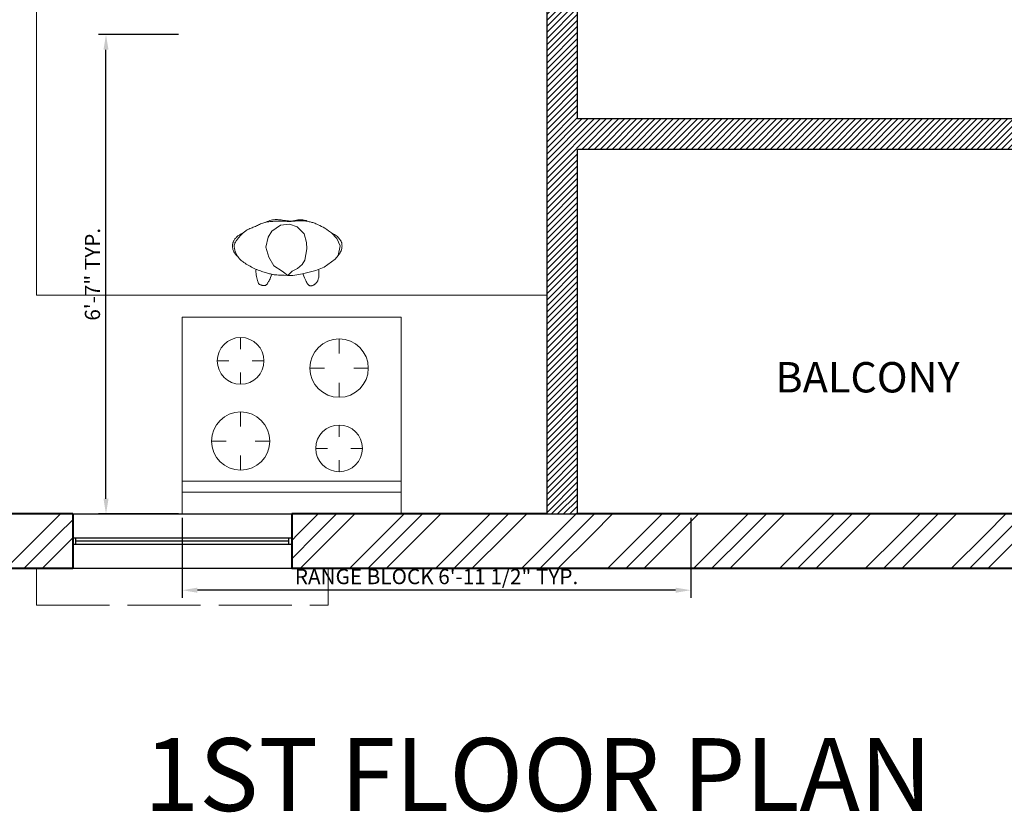
# Model space of a CAD drawing. Units: inches. Extents: x 2443635 to 2446153, y 1826255 to 1827341.
# Tile 7 of 16: x 2444366 to 2444528, y 1826821 to 1826952. Entities that reach past the tile are written whole.
import ezdxf

# ---------------------------------------------------------------- set-up
doc = ezdxf.new("R2010")
doc.units = ezdxf.units.IN
doc.linetypes.add('ACAD_ISO02W100', pattern=[15, 12, -3])
for name, color, linetype, lineweight in [('A-DIMS', 1, 'Continuous', 18), ('A-ENTG', 111, 'Continuous', 13), ('A-EQPM', 8, 'Continuous', 18), ('A-FLOR-CASE', 8, 'Continuous', 18), ('A-ROOM', 4, 'Continuous', 18), ('A-TEXT', 4, 'Continuous', 25), ('A-WALL-EXT', 7, 'Continuous', 40), ('A-WALL-INT', 9, 'Continuous', 30), ('A-WALL-OVHD', 7, 'ACAD_ISO02W100', 18), ('A-WALL-PATT', 8, 'Continuous', 13), ('A-WINDOW', 4, 'Continuous', 25)]:
    doc.layers.add(name, color=color, linetype=linetype, lineweight=lineweight)
doc.styles.add('ATT', font='romans.shx')
doc.styles.get("Standard").update_dxf_attribs({"font": 'arial.ttf'})
doc.dimstyles.new('ISO-25', dxfattribs={"dimtxt": 2.5, "dimasz": 2.5, "dimexe": 1.25, "dimexo": 0.625, "dimtad": 1, "dimlunit": 4, "dimtxsty": 'Standard', "dimcen": 2.5, "dimadec": 0, "dimazin": 0, "dimtfac": 1, "dimtmove": 0, "dimatfit": 3, "dimfxl": 1, "dimarcsym": 0})

# ---------------------------------------------------------------- blocks, each defined once
blk = doc.blocks.new('11PRNG01')
at = {"color": 0, "linetype": 'ByBlock'}
for p, q in [((0, 30), (27, 30)), ((0, 0), (0, 30)), ((3, 0), (3, 30)), ((4.5, 0), (4.5, 30)), ((27, 30), (27, 0)), ((10, 26), (10, 24)), ((21, 25.2), (21, 23.6)), ((6, 22), (8, 22)), ((14, 22), (12, 22)), ((17.8, 22), (19.4, 22)), ((24.2, 22), (22.6, 22)), ((21, 18.8), (21, 20.4)), ((10, 18), (10, 20)), ((20, 12.5), (20, 10.5)), ((9, 11.7), (9, 10.1)), ((5.8, 8.5), (7.4, 8.5)), ((12.2, 8.5), (10.6, 8.5)), ((16, 8.5), (18, 8.5)), ((24, 8.5), (22, 8.5)), ((9, 5.3), (9, 6.9)), ((20, 4.5), (20, 6.5)), ((27, 0), (0, 0))]:
    blk.add_line(p, q, dxfattribs=at)
for centre, radius in [((10, 22), 4), ((21, 22), 3.2), ((20, 8.5), 4), ((9, 8.5), 3.2)]:
    blk.add_circle(centre, radius, dxfattribs=at)
at = {"color": 0, "linetype": 'ByBlock', "style": 'ATT'}
for tag, p, flags in [('ITEM', (0, -11), 3), ('ROOM_NUMBER', (0, -20), 1), ('DEPTH', (0, -29), 3), ('WIDTH', (0, -38), 3)]:
    blk.add_attdef(tag, p, '', height=6, dxfattribs=dict(at, flags=flags))
blk = doc.blocks.new('PERSON-STANDING-PLAN')
at = {"transparency": 33554687}
for p, q in [((3.58, 9.72), (3.76, 9.79)), ((3.76, 9.79), (3.94, 9.87)), ((3.94, 9.87), (4.11, 9.95)), ((4.11, 9.95), (4.28, 10.02)), ((4.28, 10.02), (4.45, 10.1)), ((4.45, 10.1), (4.62, 10.18)), ((4.62, 10.18), (4.79, 10.25)), ((4.79, 10.25), (4.96, 10.31)), ((4.96, 10.31), (5.14, 10.38)), ((5.14, 10.38), (5.33, 10.43)), ((5.33, 10.43), (5.53, 10.48)), ((5.48, 10.5), (5.36, 10.44)), ((5.69, 10.59), (5.48, 10.5)), ((5.53, 10.48), (5.74, 10.51)), ((5.91, 10.67), (5.69, 10.59)), ((5.74, 10.51), (5.95, 10.55)), ((6.13, 10.74), (5.91, 10.67)), ((5.95, 10.55), (6.17, 10.57)), ((6.35, 10.79), (6.13, 10.74)), ((6.17, 10.57), (6.39, 10.59)), ((6.57, 10.84), (6.35, 10.79)), ((6.39, 10.59), (6.61, 10.61)), ((7.91, 9.98), (6.48, 9.01)), ((6.79, 10.87), (6.57, 10.84)), ((6.61, 10.61), (6.83, 10.62)), ((6.99, 10.89), (6.79, 10.87)), ((6.83, 10.62), (7.05, 10.63)), ((7.18, 10.9), (6.99, 10.89)), ((7.05, 10.63), (7.26, 10.64)), ((7.38, 10.9), (7.18, 10.9)), ((7.26, 10.64), (7.47, 10.65)), ((7.57, 10.88), (7.38, 10.9)), ((7.47, 10.65), (7.68, 10.65)), ((7.78, 10.87), (7.57, 10.88)), ((7.68, 10.65), (7.87, 10.65)), ((7.99, 10.84), (7.78, 10.87)), ((7.87, 10.65), (8.06, 10.65)), ((9.39, 10.13), (7.91, 9.98)), ((8.22, 10.82), (7.99, 10.84)), ((8.06, 10.65), (8.23, 10.65)), ((9.71, 10.64), (8.22, 10.82)), ((8.23, 10.65), (8.39, 10.65)), ((8.39, 10.65), (8.54, 10.64)), ((8.54, 10.64), (8.67, 10.64)), ((8.67, 10.64), (8.78, 10.63)), ((8.78, 10.63), (8.89, 10.62)), ((8.89, 10.62), (8.98, 10.61)), ((8.98, 10.61), (9.08, 10.6)), ((9.08, 10.6), (9.16, 10.59)), ((9.16, 10.59), (9.25, 10.59)), ((9.25, 10.59), (9.35, 10.59)), ((9.35, 10.59), (9.44, 10.59)), ((10.63, 9.72), (9.39, 10.13)), ((9.44, 10.59), (9.55, 10.6)), ((9.55, 10.6), (9.66, 10.61)), ((9.9, 10.69), (9.56, 10.61)), ((9.66, 10.61), (9.78, 10.62)), ((9.78, 10.62), (9.9, 10.63)), ((10.22, 10.76), (9.9, 10.69)), ((9.9, 10.63), (10.03, 10.64)), ((10.03, 10.64), (10.16, 10.66)), ((10.16, 10.66), (10.3, 10.67)), ((10.5, 10.81), (10.22, 10.76)), ((10.3, 10.67), (10.45, 10.68)), ((10.45, 10.68), (10.61, 10.7)), ((10.76, 10.84), (10.5, 10.81)), ((10.61, 10.7), (10.76, 10.71)), ((10.99, 10.86), (10.76, 10.84)), ((10.76, 10.71), (10.92, 10.71)), ((10.92, 10.71), (11.09, 10.72)), ((11.2, 10.87), (10.99, 10.86)), ((11.09, 10.72), (11.25, 10.72)), ((11.4, 10.86), (11.2, 10.87)), ((11.25, 10.72), (11.41, 10.72)), ((11.58, 10.84), (11.4, 10.86)), ((11.41, 10.72), (11.57, 10.71)), ((11.57, 10.71), (11.73, 10.7)), ((11.76, 10.81), (11.58, 10.84)), ((11.73, 10.7), (11.89, 10.68)), ((11.93, 10.77), (11.76, 10.81)), ((11.89, 10.68), (12.04, 10.67)), ((12.11, 10.73), (11.93, 10.77)), ((12.04, 10.67), (12.19, 10.64)), ((12.29, 10.67), (12.11, 10.73)), ((12.19, 10.64), (12.34, 10.62)), ((12.48, 10.61), (12.29, 10.67)), ((12.34, 10.62), (12.48, 10.59)), ((12.68, 10.55), (12.48, 10.61)), ((12.48, 10.59), (12.62, 10.56)), ((12.62, 10.56), (12.77, 10.53)), ((12.91, 10.49), (12.68, 10.55)), ((12.77, 10.53), (12.91, 10.49)), ((12.91, 10.49), (13.05, 10.45)), ((13.17, 10.43), (12.91, 10.49)), ((13.05, 10.45), (13.2, 10.41)), ((13.2, 10.41), (13.35, 10.36)), ((13.35, 10.36), (13.51, 10.3)), ((13.51, 10.3), (13.69, 10.22)), ((13.69, 10.22), (13.89, 10.14)), ((13.89, 10.14), (14.11, 10.04)), ((14.11, 10.04), (14.35, 9.93)), ((14.35, 9.93), (14.61, 9.79)), ((14.61, 9.79), (14.89, 9.64)), ((0.77, 8.12), (0.67, 8.02)), ((0.87, 8.21), (0.77, 8.12)), ((0.97, 8.29), (0.87, 8.21)), ((1.08, 8.36), (0.97, 8.29)), ((1.17, 8.42), (1.08, 8.36)), ((1.12, 8.07), (1.21, 8.17)), ((1.26, 8.47), (1.17, 8.42)), ((1.21, 8.17), (1.3, 8.27)), ((1.35, 8.51), (1.26, 8.47)), ((1.3, 8.27), (1.39, 8.37)), ((1.43, 8.54), (1.35, 8.51)), ((1.39, 8.37), (1.49, 8.47)), ((1.49, 8.56), (1.43, 8.54)), ((1.55, 8.58), (1.49, 8.56)), ((1.49, 8.47), (1.59, 8.57)), ((1.59, 8.59), (1.55, 8.58)), ((1.59, 8.57), (1.69, 8.66)), ((1.62, 8.6), (1.59, 8.59)), ((1.69, 8.66), (1.79, 8.76)), ((1.79, 8.76), (1.9, 8.85)), ((1.9, 8.85), (2.01, 8.94)), ((2.01, 8.94), (2.13, 9.02)), ((2.13, 9.02), (2.26, 9.11)), ((2.26, 9.11), (2.39, 9.19)), ((2.39, 9.19), (2.54, 9.27)), ((2.54, 9.27), (2.7, 9.35)), ((2.7, 9.35), (2.86, 9.42)), ((2.86, 9.42), (3.04, 9.5)), ((3.04, 9.5), (3.21, 9.57)), ((3.21, 9.57), (3.39, 9.65)), ((3.39, 9.65), (3.58, 9.72)), ((6.48, 9.01), (5.88, 8.02)), ((11.79, 8.58), (10.63, 9.72)), ((12.18, 7.14), (11.79, 8.58)), ((14.89, 9.64), (15.18, 9.47)), ((15.18, 9.47), (15.49, 9.28)), ((15.49, 9.28), (15.8, 9.07)), ((15.8, 9.07), (16.12, 8.84)), ((16.12, 8.84), (16.44, 8.59)), ((16.26, 8.74), (17.17, 7.78)), ((16.44, 8.59), (16.61, 8.53)), ((16.61, 8.53), (16.77, 8.45)), ((16.77, 8.45), (16.94, 8.35)), ((16.94, 8.35), (17.1, 8.23)), ((17.1, 8.23), (17.24, 8.1)), ((0.01, 6.79), (0, 6.71)), ((0, 6.71), (0, 6.61)), ((0, 6.61), (0, 6.52)), ((0, 6.52), (0, 6.42)), ((0.02, 6.88), (0.01, 6.79)), ((0.04, 6.97), (0.02, 6.88)), ((0.06, 7.06), (0.04, 6.97)), ((0.08, 7.15), (0.06, 7.06)), ((0.11, 7.23), (0.08, 7.15)), ((0.15, 7.33), (0.11, 7.23)), ((0.2, 7.42), (0.15, 7.33)), ((0.25, 7.51), (0.2, 7.42)), ((0.32, 7.61), (0.25, 7.51)), ((0.28, 6.52), (0.29, 6.66)), ((0.29, 6.38), (0.28, 6.52)), ((0.29, 6.66), (0.31, 6.8)), ((0.31, 6.8), (0.35, 6.93)), ((0.39, 7.71), (0.32, 7.61)), ((0.35, 6.93), (0.4, 7.06)), ((0.48, 7.82), (0.39, 7.71)), ((0.4, 7.06), (0.46, 7.18)), ((0.46, 7.18), (0.52, 7.3)), ((0.57, 7.92), (0.48, 7.82)), ((0.52, 7.3), (0.6, 7.41)), ((0.67, 8.02), (0.57, 7.92)), ((0.6, 7.41), (0.68, 7.53)), ((0.68, 7.53), (0.76, 7.64)), ((0.76, 7.64), (0.85, 7.75)), ((0.85, 7.75), (0.94, 7.85)), ((0.94, 7.85), (1.03, 7.96)), ((1.03, 7.96), (1.12, 8.07)), ((5.88, 8.02), (5.48, 6.38)), ((12.22, 6.07), (12.18, 7.14)), ((17.17, 7.78), (17.68, 6.58)), ((17.24, 8.1), (17.38, 7.96)), ((17.68, 6.58), (17.36, 5.01)), ((17.38, 7.96), (17.51, 7.82)), ((17.51, 7.82), (17.61, 7.69)), ((17.61, 7.69), (17.7, 7.56)), ((17.7, 7.56), (17.78, 7.45)), ((17.78, 7.45), (17.84, 7.34)), ((17.84, 7.34), (17.88, 7.24)), ((17.88, 7.24), (17.92, 7.15)), ((17.92, 7.15), (17.95, 7.06)), ((17.95, 7.06), (17.97, 6.97)), ((17.97, 6.97), (17.98, 6.88)), ((17.98, 6.88), (17.99, 6.79)), ((17.99, 6.79), (18, 6.71)), ((18, 6.71), (18.01, 6.61)), ((18.01, 6.52), (18, 6.42)), ((18.01, 6.61), (18.01, 6.52)), ((0, 6.42), (0.01, 6.33)), ((0.01, 6.33), (0.02, 6.22)), ((0.02, 6.22), (0.04, 6.12)), ((0.04, 6.12), (0.06, 6)), ((0.06, 6), (0.1, 5.88)), ((0.1, 5.88), (0.15, 5.75)), ((0.15, 5.75), (0.23, 5.6)), ((0.23, 5.6), (0.33, 5.43)), ((0.3, 6.24), (0.29, 6.38)), ((0.32, 6.09), (0.3, 6.24)), ((0.35, 5.95), (0.32, 6.09)), ((0.33, 5.43), (0.48, 5.23)), ((0.39, 5.81), (0.35, 5.95)), ((0.43, 5.68), (0.39, 5.81)), ((0.48, 5.55), (0.43, 5.68)), ((0.53, 5.42), (0.48, 5.55)), ((0.48, 5.23), (0.67, 5.01)), ((0.58, 5.3), (0.53, 5.42)), ((0.64, 5.19), (0.58, 5.3)), ((0.7, 5.07), (0.64, 5.19)), ((0.67, 5.01), (0.91, 4.75)), ((0.77, 4.96), (0.7, 5.07)), ((0.85, 4.85), (0.77, 4.96)), ((5.48, 6.38), (5.95, 4.72)), ((11.9, 4.25), (12.22, 6.07)), ((17.36, 5.01), (16.88, 4.4)), ((17.36, 5), (17.14, 4.74)), ((17.54, 5.23), (17.36, 5)), ((17.68, 5.42), (17.54, 5.23)), ((17.78, 5.6), (17.68, 5.42)), ((17.86, 5.75), (17.78, 5.6)), ((17.91, 5.88), (17.86, 5.75)), ((17.94, 6), (17.91, 5.88)), ((17.96, 6.12), (17.94, 6)), ((17.98, 6.22), (17.96, 6.12)), ((17.99, 6.33), (17.98, 6.22)), ((18, 6.42), (17.99, 6.33)), ((0.93, 4.74), (0.85, 4.85)), ((1.01, 4.63), (0.93, 4.74)), ((1.1, 4.52), (1.01, 4.63)), ((1.21, 4.41), (1.1, 4.52)), ((1.32, 4.3), (1.21, 4.41)), ((1.44, 4.19), (1.32, 4.3)), ((1.57, 4.08), (1.44, 4.19)), ((1.72, 3.96), (1.57, 4.08)), ((1.88, 3.84), (1.72, 3.96)), ((2.06, 3.71), (1.88, 3.84)), ((2.26, 3.59), (2.06, 3.71)), ((2.46, 3.46), (2.26, 3.59)), ((2.67, 3.34), (2.46, 3.46)), ((2.89, 3.21), (2.67, 3.34)), ((5.95, 4.72), (6.81, 3.29)), ((6.81, 3.29), (8.17, 2.41)), ((10.66, 2.88), (11.44, 3.53)), ((11.44, 3.53), (11.9, 4.25)), ((16.88, 4.4), (15.08, 3.08)), ((3.11, 3.09), (2.89, 3.21)), ((3.33, 2.98), (3.11, 3.09)), ((3.56, 2.87), (3.33, 2.98)), ((3.77, 2.77), (3.56, 2.87)), ((3.99, 2.68), (3.77, 2.77)), ((3.86, 2.7), (3.84, 2.5)), ((3.84, 2.5), (3.84, 2.27)), ((3.84, 2.27), (3.86, 2.03)), ((3.86, 2.03), (3.89, 1.79)), ((3.89, 1.79), (3.93, 1.54)), ((4.2, 2.6), (3.99, 2.68)), ((4.4, 2.52), (4.2, 2.6)), ((4.6, 2.45), (4.4, 2.52)), ((4.8, 2.38), (4.6, 2.45)), ((5, 2.32), (4.8, 2.38)), ((5.19, 2.26), (5, 2.32)), ((5.38, 2.2), (5.19, 2.26)), ((5.56, 2.15), (5.38, 2.2)), ((5.74, 2.09), (5.56, 2.15)), ((5.92, 2.05), (5.74, 2.09)), ((6.09, 2), (5.92, 2.05)), ((6.25, 1.96), (6.09, 2)), ((6.41, 1.92), (6.25, 1.96)), ((6.26, 1.39), (6.36, 1.65)), ((6.36, 1.65), (6.46, 1.91)), ((6.55, 1.89), (6.41, 1.92)), ((6.7, 1.86), (6.55, 1.89)), ((6.85, 1.83), (6.7, 1.86)), ((7.04, 1.81), (6.85, 1.83)), ((7.27, 1.79), (7.04, 1.81)), ((7.57, 1.77), (7.27, 1.79)), ((7.97, 1.75), (7.57, 1.77)), ((8.47, 1.73), (7.97, 1.75)), ((8.17, 2.41), (9.1, 1.71)), ((9.1, 1.71), (8.47, 1.73)), ((9.1, 1.71), (9.82, 2.41)), ((9.89, 1.71), (9.1, 1.71)), ((9.82, 2.41), (10.66, 2.88)), ((11.53, 1.95), (9.89, 1.71)), ((13.68, 2.54), (11.53, 1.95)), ((11.63, 1.91), (11.74, 1.61)), ((15.08, 3.08), (13.68, 2.54)), ((14.17, 2.51), (14.14, 2.7)), ((14.19, 2.34), (14.17, 2.51)), ((14.2, 2.16), (14.19, 2.34)), ((14.19, 1.54), (14.2, 1.68)), ((14.21, 2), (14.2, 2.16)), ((14.2, 1.68), (14.21, 1.83)), ((14.21, 1.83), (14.21, 2)), ((3.93, 1.54), (3.98, 1.3)), ((3.98, 1.3), (4.03, 1.08)), ((4.03, 1.08), (4.09, 0.89)), ((4.09, 0.89), (4.14, 0.73)), ((4.14, 0.73), (4.19, 0.59)), ((4.19, 0.59), (4.24, 0.49)), ((4.24, 0.49), (4.29, 0.4)), ((4.29, 0.4), (4.34, 0.34)), ((4.34, 0.34), (4.39, 0.28)), ((4.39, 0.28), (4.45, 0.24)), ((4.45, 0.24), (4.51, 0.2)), ((4.51, 0.2), (4.57, 0.17)), ((4.57, 0.17), (4.64, 0.14)), ((4.64, 0.14), (4.72, 0.11)), ((4.72, 0.11), (4.79, 0.09)), ((4.79, 0.09), (4.86, 0.07)), ((4.86, 0.07), (4.93, 0.05)), ((4.93, 0.05), (5, 0.04)), ((5, 0.04), (5.07, 0.03)), ((5.07, 0.03), (5.13, 0.03)), ((5.13, 0.03), (5.19, 0.03)), ((5.19, 0.03), (5.24, 0.03)), ((5.24, 0.03), (5.29, 0.04)), ((5.29, 0.04), (5.34, 0.05)), ((5.34, 0.05), (5.39, 0.06)), ((5.39, 0.06), (5.43, 0.08)), ((5.43, 0.08), (5.47, 0.11)), ((5.47, 0.11), (5.51, 0.13)), ((5.51, 0.13), (5.55, 0.16)), ((5.55, 0.16), (5.59, 0.2)), ((5.59, 0.2), (5.63, 0.24)), ((5.63, 0.24), (5.68, 0.29)), ((5.68, 0.29), (5.72, 0.35)), ((5.72, 0.35), (5.77, 0.42)), ((5.77, 0.42), (5.82, 0.5)), ((5.82, 0.5), (5.88, 0.59)), ((5.88, 0.59), (5.94, 0.7)), ((5.94, 0.7), (6.01, 0.83)), ((6.01, 0.83), (6.09, 0.99)), ((6.09, 0.99), (6.17, 1.17)), ((6.17, 1.17), (6.26, 1.39)), ((11.74, 1.61), (11.85, 1.34)), ((11.85, 1.34), (11.95, 1.1)), ((11.95, 1.1), (12.05, 0.89)), ((12.05, 0.89), (12.13, 0.71)), ((12.13, 0.71), (12.22, 0.55)), ((12.22, 0.55), (12.29, 0.41)), ((12.29, 0.41), (12.37, 0.3)), ((12.37, 0.3), (12.44, 0.21)), ((12.44, 0.21), (12.51, 0.14)), ((12.51, 0.14), (12.58, 0.08)), ((12.58, 0.08), (12.64, 0.04)), ((12.64, 0.04), (12.71, 0.02)), ((12.71, 0.02), (12.77, 0.01)), ((12.77, 0.01), (12.84, 0)), ((12.84, 0), (12.9, 0)), ((12.9, 0), (12.97, 0.01)), ((12.97, 0.01), (13.03, 0.02)), ((13.03, 0.02), (13.1, 0.04)), ((13.1, 0.04), (13.17, 0.06)), ((13.17, 0.06), (13.24, 0.09)), ((13.24, 0.09), (13.3, 0.12)), ((13.3, 0.12), (13.37, 0.15)), ((13.37, 0.15), (13.43, 0.18)), ((13.43, 0.18), (13.49, 0.22)), ((13.49, 0.22), (13.55, 0.26)), ((13.55, 0.26), (13.61, 0.31)), ((13.61, 0.31), (13.67, 0.35)), ((13.67, 0.35), (13.72, 0.41)), ((13.72, 0.41), (13.77, 0.47)), ((13.77, 0.47), (13.82, 0.53)), ((13.82, 0.53), (13.87, 0.6)), ((13.87, 0.6), (13.92, 0.67)), ((13.92, 0.67), (13.96, 0.75)), ((13.96, 0.75), (14.01, 0.84)), ((14.01, 0.84), (14.05, 0.94)), ((14.05, 0.94), (14.08, 1.04)), ((14.08, 1.04), (14.11, 1.15)), ((14.11, 1.15), (14.14, 1.27)), ((14.14, 1.27), (14.17, 1.4)), ((14.17, 1.4), (14.19, 1.54))]:
    blk.add_line(p, q, dxfattribs=at)
blk = doc.blocks.new('BASE-CABINET-L-PLAN')
at = {"transparency": 33554687}
for p, q in [((0, 78), (36, 78)), ((36, 0), (36, 78)), ((120, 0), (36, 0))]:
    blk.add_line(p, q, dxfattribs=at)
blk = doc.blocks.new('WIN-36-PLAN')
at = {"transparency": 33554687}
for p, q in [((0, 9), (36, 9)), ((0, 0), (0, 9)), ((36, 9), (36, 0)), ((0, 5), (36, 5)), ((0.5, 4), (0.5, 5)), ((35.5, 5), (35.5, 4)), ((0, 4), (36, 4)), ((0.5, 4.5), (35.5, 4.5)), ((36, 0), (0, 0))]:
    blk.add_line(p, q, dxfattribs=at)
blk = doc.blocks.new('WINDOW-HOOD-48-PLAN')
at = {"transparency": 33554687}
for p, q in [((0, 6), (0, 0)), ((48, 0), (48, 6)), ((0, 0), (48, 0))]:
    blk.add_line(p, q, dxfattribs=at)
blk = doc.blocks.new('*D68')
at = {"layer": 'A-DIMS', "color": 0, "lineweight": -2, "transparency": 16777216}
for p, q in [((2444392.55, 1826869.66), (2444392.55, 1826856.49)), ((2444476.21, 1826869.66), (2444476.21, 1826856.49)), ((2444473.71, 1826857.74), (2444395.05, 1826857.74))]:
    blk.add_line(p, q, dxfattribs=at)
at = {"layer": 'A-DIMS', "color": 0, "transparency": 16777216}
for points in [[(2444395.05, 1826858.16), (2444395.05, 1826857.32), (2444392.55, 1826857.74)], [(2444473.71, 1826858.16), (2444473.71, 1826857.32), (2444476.21, 1826857.74)]]:
    blk.add_solid(points, dxfattribs=at)
at = {"layer": 'Defpoints', "color": 0, "transparency": 16777216}
for p in [(2444392.55, 1826870.29), (2444476.21, 1826870.29), (2444392.55, 1826857.74)]:
    blk.add_point(p, dxfattribs=at)
at = {"layer": 'A-DIMS', "color": 0, "transparency": 16777216, "insert": (2444434.38, 1826859.66), "char_height": 2.5, "attachment_point": 5}
blk.add_mtext('RANGE BLOCK 6\'-11 1/2" TYP.', dxfattribs=at)
blk = doc.blocks.new('*D69')
at = {"layer": 'A-DIMS', "color": 0, "lineweight": -2, "transparency": 16777216}
for p, q in [((2444391.93, 1826949.17), (2444378.75, 1826949.17)), ((2444380, 1826872.79), (2444380, 1826946.67)), ((2444391.93, 1826870.29), (2444378.75, 1826870.29))]:
    blk.add_line(p, q, dxfattribs=at)
at = {"layer": 'A-DIMS', "color": 0, "transparency": 16777216}
for points in [[(2444379.59, 1826946.67), (2444380.42, 1826946.67), (2444380, 1826949.17)], [(2444379.59, 1826872.79), (2444380.42, 1826872.79), (2444380, 1826870.29)]]:
    blk.add_solid(points, dxfattribs=at)
at = {"layer": 'Defpoints', "color": 0, "transparency": 16777216}
for p in [(2444380, 1826949.17), (2444392.55, 1826949.17), (2444392.55, 1826870.29)]:
    blk.add_point(p, dxfattribs=at)
at = {"layer": 'A-DIMS', "color": 0, "transparency": 16777216, "insert": (2444378.1, 1826909.73), "char_height": 2.5, "attachment_point": 5, "rotation": 90}
blk.add_mtext('6\'-7" TYP.', dxfattribs=at)

msp = doc.modelspace()

# ---------------------------------------------------------------- hatches: boundary and pattern name
at = {"layer": 'A-WALL-PATT'}
h = msp.add_hatch(dxfattribs=at)
h.set_pattern_fill('GOST_GROUND', color=256)
h.paths.add_polyline_path([(2444332.553, 1827147.288), (2444332.553, 1827152.288), (2444332.553, 1827161.288), (2444328.953, 1827161.288), (2444323.553, 1827161.288), (2444323.553, 1826984.288), (2444332.553, 1826984.288), (2444332.553, 1827062.288), (2444332.553, 1827067.288)])
h.paths.add_polyline_path([(2444332.553, 1826948.288), (2444323.553, 1826948.288), (2444323.553, 1826861.288), (2444374.553, 1826861.288), (2444374.553, 1826870.288), (2444332.553, 1826870.288)])
h.paths.add_polyline_path([(2444647.553, 1826941.288), (2444638.553, 1826941.288), (2444638.553, 1826935.288), (2444638.553, 1826930.288), (2444638.553, 1826870.288), (2444457.553, 1826870.288), (2444452.553, 1826870.288), (2444410.553, 1826870.288), (2444410.553, 1826861.288), (2444647.553, 1826861.288)])
h.paths.add_polyline_path([(2444647.553, 1827161.288), (2444638.553, 1827161.288), (2444638.553, 1827152.288), (2444638.553, 1827147.288), (2444638.553, 1826989.288), (2444647.553, 1826989.288)])
h.paths.add_polyline_path([(2444647.553, 1827305.288), (2444494.553, 1827305.288), (2444494.553, 1827296.288), (2444498.051, 1827296.288), (2444638.553, 1827296.288), (2444638.553, 1827254.288), (2444647.553, 1827254.288)])
h.paths.add_polyline_path([(2444476.553, 1827305.288), (2444323.553, 1827305.288), (2444323.553, 1827254.288), (2444332.553, 1827254.288), (2444332.553, 1827296.288), (2444346.141, 1827296.288), (2444476.553, 1827296.288)])
h.paths.add_polyline_path([(2444323.553, 1827305.288), (2444282.553, 1827305.288), (2444282.553, 1827147.459), (2444323.553, 1827147.459), (2444323.553, 1827152.459), (2444287.553, 1827152.459), (2444287.553, 1827300.288), (2444323.553, 1827300.288)])
h.paths.add_polyline_path([(2444688.553, 1827305.288), (2444647.553, 1827305.288), (2444647.553, 1827300.288), (2444683.553, 1827300.288), (2444683.553, 1827152.362), (2444647.553, 1827152.362), (2444647.553, 1827147.362), (2444688.553, 1827147.362)])
h = msp.add_hatch(dxfattribs=at)
h.set_pattern_fill('JIS_WOOD', color=256)
h.paths.add_polyline_path([(2444481.553, 1827095.288), (2444476.553, 1827095.288), (2444476.553, 1827067.288), (2444332.553, 1827067.288), (2444332.553, 1827062.288), (2444481.553, 1827062.288)])
h.paths.add_polyline_path([(2444457.553, 1827020.288), (2444452.553, 1827020.288), (2444452.553, 1826870.288), (2444457.553, 1826870.288), (2444457.553, 1826930.288), (2444530.053, 1826930.288), (2444530.053, 1826935.288), (2444457.553, 1826935.288)])
h.paths.add_polyline_path([(2444457.553, 1827062.288), (2444452.553, 1827062.288), (2444452.553, 1827056.288), (2444457.553, 1827056.288)])
h.paths.add_polyline_path([(2444638.553, 1826935.288), (2444566.053, 1826935.288), (2444566.053, 1826930.288), (2444638.553, 1826930.288)])
h.paths.add_polyline_path([(2444638.553, 1827152.288), (2444518.553, 1827152.288), (2444518.553, 1827156.288), (2444513.553, 1827156.288), (2444513.553, 1827147.288), (2444638.553, 1827147.288)])
h.paths.add_polyline_path([(2444518.553, 1827296.288), (2444513.553, 1827296.288), (2444513.553, 1827224.288), (2444507.553, 1827224.288), (2444507.553, 1827223.788), (2444507.553, 1827219.288), (2444513.553, 1827219.288), (2444513.553, 1827192.288), (2444518.553, 1827192.288)])
h.paths.add_polyline_path([(2444477.553, 1827223.788, -0.0041669), (2444477.557, 1827224.288), (2444457.553, 1827224.288), (2444457.553, 1827296.288), (2444452.553, 1827296.288), (2444452.553, 1827192.288), (2444457.553, 1827192.288), (2444457.553, 1827219.288), (2444477.553, 1827219.288)])
h.paths.add_polyline_path([(2444481.553, 1827152.288), (2444332.553, 1827152.288), (2444332.553, 1827147.288), (2444476.553, 1827147.288), (2444476.553, 1827137.288), (2444481.553, 1827137.288)])

# ---------------------------------------------------------------- linework, layer by layer
at = {"layer": 'A-WALL-EXT'}
for p, q in [((2444374.553, 1826870.288), (2444332.553, 1826870.288)), ((2444374.553, 1826870.288), (2444374.553, 1826861.288)), ((2444452.553, 1826870.288), (2444410.553, 1826870.288)), ((2444410.553, 1826870.288), (2444410.553, 1826861.288)), ((2444638.553, 1826870.288), (2444457.553, 1826870.288)), ((2444374.553, 1826861.288), (2444323.553, 1826861.288)), ((2444647.553, 1826861.288), (2444410.553, 1826861.288))]:
    msp.add_line(p, q, dxfattribs=at)
at = {"layer": 'A-WALL-INT'}
for p, q in [((2444452.553, 1826870.288), (2444452.553, 1827020.288)), ((2444457.553, 1826935.288), (2444457.553, 1827020.288)), ((2444530.053, 1826935.288), (2444457.553, 1826935.288)), ((2444457.553, 1826870.288), (2444457.553, 1826930.288)), ((2444530.053, 1826930.288), (2444457.553, 1826930.288)), ((2444452.553, 1826870.288), (2444457.553, 1826870.288))]:
    msp.add_line(p, q, dxfattribs=at)
at = {"layer": 'A-WINDOW'}
for p, q in [((2444374.553, 1826861.288), (2444374.553, 1826870.288)), ((2444410.553, 1826870.288), (2444410.553, 1826861.288))]:
    msp.add_line(p, q, dxfattribs=at)

# ---------------------------------------------------------------- block references
at = {"layer": 'A-ENTG', "transparency": 33554687}
msp.add_blockref('PERSON-STANDING-PLAN', (2444400.822, 1826907.83), dxfattribs=at)
at = {"layer": 'A-EQPM', "xscale": 1.199999999999791, "yscale": 1.199999999999791, "zscale": 1.199999999999791, "rotation": 89.99999999999999}
msp.add_blockref('11PRNG01', (2444428.553, 1826870.288), dxfattribs=at)
at = {"layer": 'A-FLOR-CASE', "transparency": 33554687}
msp.add_blockref('BASE-CABINET-L-PLAN', (2444332.553, 1826906.288), dxfattribs=at)
at = {"layer": 'A-WALL-OVHD', "transparency": 33554687}
msp.add_blockref('WINDOW-HOOD-48-PLAN', (2444368.553, 1826855.288), dxfattribs=at)
at = {"layer": 'A-WINDOW', "transparency": 33554687, "rotation": 180}
msp.add_blockref('WIN-36-PLAN', (2444410.552, 1826870.288), dxfattribs=at)

# ---------------------------------------------------------------- texts
at = {"layer": 'A-ROOM', "insert": (2444490.132, 1826895.283), "char_height": 5, "attachment_point": 1}
msp.add_mtext_dynamic_manual_height_columns('BALCONY', width=52.37406, gutter_width=12.5, heights=[0], dxfattribs=at)
at = {"layer": 'A-TEXT', "insert": (2444386.234, 1826833.401), "char_height": 12, "attachment_point": 1}
msp.add_mtext_dynamic_manual_height_columns('1ST FLOOR PLAN', width=201.69861, gutter_width=12.5, heights=[0], dxfattribs=at)

# ---------------------------------------------------------------- dimensions: what is measured, and where the dimension line sits
at = {"layer": 'A-DIMS', "transparency": 33554687}
for base, p1, p2, angle, text, picture, middle in [((2444380.004, 1826949.175), (2444392.553, 1826870.288), (2444392.553, 1826949.175), 90, '<> TYP.', '*D69', (2444378.103, 1826909.731)), ((2444392.553, 1826857.74), (2444476.207, 1826870.288), (2444392.553, 1826870.288), 180, 'RANGE BLOCK <> TYP.', '*D68', (2444434.38, 1826859.658))]:
    dim = msp.add_linear_dim(base=base, p1=p1, p2=p2, angle=angle, text=text, dimstyle='ISO-25', override={"dimdec": 1, "dimlfac": 1, "dimrnd": 0, "dimzin": 1, "dimdsep": 46, "dimlunit": 4, "dimfrac": 2}, dxfattribs=at)
    dim.commit()
    dim.dimension.update_dxf_attribs({"geometry": picture, "text_midpoint": middle})

doc.saveas('drawing.dxf')
